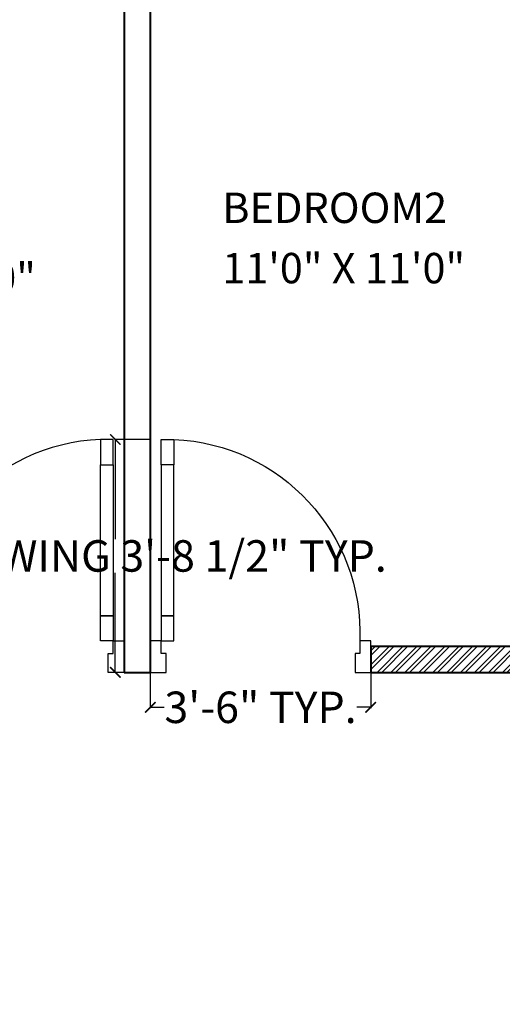
# Model space of a CAD drawing. Units: inches. Extents: x 528 to 2520, y -151 to 1354.
# Tile 8 of 41: x 720 to 812, y 1043 to 1231. Entities that reach past the tile are written whole.
import ezdxf

# ---------------------------------------------------------------- set-up
doc = ezdxf.new("R2010")
doc.units = ezdxf.units.IN
doc.header["$MEASUREMENT"] = 0
for name, color, linetype, lineweight in [('A-ANNO-DIMS', 2, 'Continuous', 18), ('A-AREA-IDEN', 7, 'Continuous', 18), ('A-Door', 150, 'Continuous', 25), ('A-WALL-PATT', 6, 'Continuous', 13), ('walls', 7, 'Continuous', 40)]:
    doc.layers.add(name, color=color, linetype=linetype, lineweight=lineweight)
doc.layers.add('NT', color=1, linetype='Continuous')
doc.styles.get("Standard").update_dxf_attribs({"font": 'arial.ttf'})
doc.dimstyles.get("Standard").update_dxf_attribs({"dimtxt": 6, "dimasz": 2, "dimexe": 0.18, "dimexo": 0.0625, "dimgap": 0.09, "dimtad": 0, "dimtih": 1, "dimtoh": 1, "dimdec": 1, "dimzin": 0, "dimdsep": 46, "dimlunit": 3, "dimtxsty": 'Standard', "dimblk": 'ARCHTICK', "dimcen": 0.09, "dimadec": 0, "dimazin": 0, "dimtfac": 1, "dimtdec": 1, "dimtofl": 0, "dimtmove": 0, "dimatfit": 3, "dimfxl": 1, "dimtolj": 1, "dimtzin": 0, "dimarcsym": 0})

# ---------------------------------------------------------------- blocks, each defined once
blk = doc.blocks.new('A$C7DB75F4D')
at = {"layer": 'A-Door'}
for points in [[(625, 740), (625, 660), (665, 660), (665, 740)], [(625, 180), (625, 660), (665, 660), (665, 180)], [(625, 100), (625, 180), (665, 180), (665, 100)], [(35, 100), (35, 60), (50, 60), (50, 50), (50, 0), (0, 0), (0, 100)], [(665, 100), (700, 100), (700, 0), (650, 0), (650, 50), (650, 60), (665, 60)]]:
    blk.add_lwpolyline(points, close=True, dxfattribs=at)
at = {"layer": 'NT'}
blk.add_arc((650, 125), 615.5, 92.3278, 182.3278, dxfattribs=at)
blk = doc.blocks.new('_ArchTick')
at = {"color": 0, "linetype": 'ByBlock', "const_width": 0.15}
blk.add_lwpolyline([(-0.5, -0.5), (0.5, 0.5)], dxfattribs=at)
blk = doc.blocks.new('*D40')
at = {"layer": 'A-ANNO-DIMS', "color": 0, "lineweight": -2, "transparency": 16777216}
for p, q in [((744.63, 1150.5), (737.86, 1150.5)), ((738.04, 1150.5), (738.04, 1131.5)), ((738.04, 1106.1), (738.04, 1125.11)), ((744.63, 1106.1), (737.86, 1106.1))]:
    blk.add_line(p, q, dxfattribs=at)
at = {"layer": 'Defpoints', "color": 0, "transparency": 16777216}
for p in [(738.04, 1150.5), (744.7, 1150.5), (744.7, 1106.1)]:
    blk.add_point(p, dxfattribs=at)
at = {"layer": 'A-ANNO-DIMS', "color": 0, "lineweight": -2, "transparency": 16777216, "xscale": 2, "yscale": 2, "zscale": 2}
for p, rotation in [((738.04, 1150.5), 90), ((738.04, 1106.1), 270)]:
    blk.add_blockref('_ArchTick', p, dxfattribs=dict(at, rotation=rotation))
at = {"layer": 'A-ANNO-DIMS', "color": 0, "transparency": 16777216, "insert": (738.04, 1128.3), "char_height": 6, "attachment_point": 5}
blk.add_mtext('\\A1;DOOR SWING 3\'-8 1/2" TYP.', dxfattribs=at)
blk = doc.blocks.new('*D41')
at = {"layer": 'A-ANNO-DIMS', "color": 0, "lineweight": -2, "transparency": 16777216}
for p, q in [((744.7, 1106.04), (744.7, 1099.26)), ((786.7, 1106.04), (786.7, 1099.26)), ((744.7, 1099.44), (747.32, 1099.44)), ((786.7, 1099.44), (784.07, 1099.44))]:
    blk.add_line(p, q, dxfattribs=at)
at = {"layer": 'Defpoints', "color": 0, "transparency": 16777216}
for p in [(744.7, 1106.1), (786.7, 1106.1), (744.7, 1099.44)]:
    blk.add_point(p, dxfattribs=at)
at = {"layer": 'A-ANNO-DIMS', "color": 0, "lineweight": -2, "transparency": 16777216, "xscale": 2, "yscale": 2, "zscale": 2, "rotation": 180}
blk.add_blockref('_ArchTick', (744.7, 1099.44), dxfattribs=at)
at = {"layer": 'A-ANNO-DIMS', "color": 0, "lineweight": -2, "transparency": 16777216, "xscale": 2, "yscale": 2, "zscale": 2}
blk.add_blockref('_ArchTick', (786.7, 1099.44), dxfattribs=at)
at = {"layer": 'A-ANNO-DIMS', "color": 0, "transparency": 16777216, "insert": (765.7, 1099.44), "char_height": 6, "attachment_point": 5}
blk.add_mtext('\\A1;3\'-6" TYP.', dxfattribs=at)

msp = doc.modelspace()

# ---------------------------------------------------------------- hatches: boundary and pattern name
at = {"layer": 'A-WALL-PATT'}
h = msp.add_hatch(dxfattribs=at)
h.set_pattern_fill('ANSI32', color=256, scale=5)
h.paths.add_polyline_path([(595.7, 1163.86), (586.7, 1163.86), (586.7, 969.1), (598.24, 969.1), (603.24, 969.1), (603.24, 974.1), (595.7, 974.1), (595.7, 1082.1), (691.7, 1082.1), (691.7, 1087.1), (691.7, 1106.1), (697.7, 1106.1), (697.7, 1111.1), (686.7, 1111.1), (686.7, 1087.1), (595.7, 1087.1)])
h.paths.add_polyline_path([(688.7, 974.1), (651.24, 974.1), (651.24, 969.1), (688.7, 969.1)])
h.paths.add_polyline_path([(885.7, 1171.37), (876.7, 1171.37), (876.7, 1111.1), (786.7, 1111.1), (786.7, 1106.1), (876.7, 1106.1), (876.7, 974.1), (786.7, 974.1), (786.7, 969.1), (876.7, 969.1), (876.7, 825.1), (834.7, 825.1), (834.7, 816.1), (885.7, 816.1)])
h.paths.add_polyline_path([(885.7, 1317.1), (876.65, 1317.1), (876.65, 1308.1), (876.7, 1308.1), (876.7, 1248.1), (822.7, 1248.1), (822.7, 1243.1), (876.7, 1243.1), (876.7, 1219.37), (885.7, 1219.37)])
h.paths.add_polyline_path([(852.65, 1317.1), (787.7, 1317.1), (787.7, 1248.1), (784.26, 1248.1), (784.26, 1243.1), (792.7, 1243.1), (792.7, 1249.1), (792.7, 1308.1), (852.65, 1308.1)])
h.paths.add_polyline_path([(684.7, 1317.1), (619.7, 1317.1), (619.7, 1308.1), (679.7, 1308.1), (679.7, 1248.1), (679.7, 1243.1), (684.7, 1243.1), (684.7, 1248.25)])
h.paths.add_polyline_path([(595.7, 1308.1), (595.7, 1317.1), (586.7, 1317.1), (586.7, 1211.86), (595.7, 1211.86), (595.7, 1243.1), (649.7, 1243.1), (649.7, 1248.1), (595.7, 1248.1)])
h.paths.add_polyline_path([(744.7, 969.1), (744.7, 974.1), (724.7, 974.1), (724.7, 969.1), (739.7, 969.1), (739.7, 874.29), (744.7, 874.29)])
h.paths.add_polyline_path([(739.7, 969.1), (727.7, 969.1), (727.7, 965.12), (730.74, 965.12), (730.74, 961.68), (734.43, 961.68), (734.43, 957.24), (739.7, 957.24)], flags=17)
h.paths.add_polyline_path([(786.7, 825.1), (744.7, 825.1), (744.7, 832.29), (739.7, 832.29), (739.7, 816.1), (786.7, 816.1)])

# ---------------------------------------------------------------- linework, layer by layer
at = {"layer": 'walls'}
for p, q in [((739.7, 1243.1), (739.7, 1111.1)), ((744.7, 1243.1), (744.7, 1111.1)), ((739.7, 1111.1), (739.7, 1106.1)), ((744.7, 1111.1), (744.7, 1106.1)), ((786.7, 1111.1), (876.7, 1111.1)), ((786.7, 1111.1), (786.7, 1106.1)), ((739.7, 1106.1), (744.7, 1106.1)), ((786.7, 1106.1), (876.7, 1106.1))]:
    msp.add_line(p, q, dxfattribs=at)

# ---------------------------------------------------------------- block references
at = {"layer": 'A-Door', "yscale": 0.0600000000000059, "zscale": 0.0600000000000059}
for p, xscale in [((697.7, 1106.1), 0.0600000000000059), ((786.7, 1106.1), -0.0600000000000059)]:
    msp.add_blockref('A$C7DB75F4D', p, dxfattribs=dict(at, xscale=xscale))

# ---------------------------------------------------------------- texts
at = {"layer": 'A-AREA-IDEN'}
for s, height, p in [('BEDROOM2', 5.793, (758.41, 1191.78)), ('11\'0" X 11\'0"', 5.7926, (758.41, 1180.28)), ('12\'0" X 11\'0"', 5.7926, (676.64, 1178.46))]:
    msp.add_text(s, height=height, dxfattribs=at).set_placement(p)

# ---------------------------------------------------------------- dimensions: what is measured, and where the dimension line sits
at = {"layer": 'A-ANNO-DIMS'}
for base, p1, p2, angle, text, picture, middle in [((738.04, 1150.5), (744.7, 1106.1), (744.7, 1150.5), 90, 'DOOR SWING <> TYP.', '*D40', (738.04, 1128.3)), ((744.7, 1099.44), (786.7, 1106.1), (744.7, 1106.1), 180, '<> TYP.', '*D41', (765.7, 1099.44))]:
    dim = msp.add_linear_dim(base=base, p1=p1, p2=p2, angle=angle, text=text, dimstyle='Standard', override={"dimdec": 1, "dimlfac": 1, "dimrnd": 0, "dimzin": 1, "dimdsep": 46, "dimlunit": 4, "dimfrac": 2}, dxfattribs=at)
    dim.commit()
    dim.dimension.update_dxf_attribs({"geometry": picture, "text_midpoint": middle})

doc.saveas('drawing.dxf')
